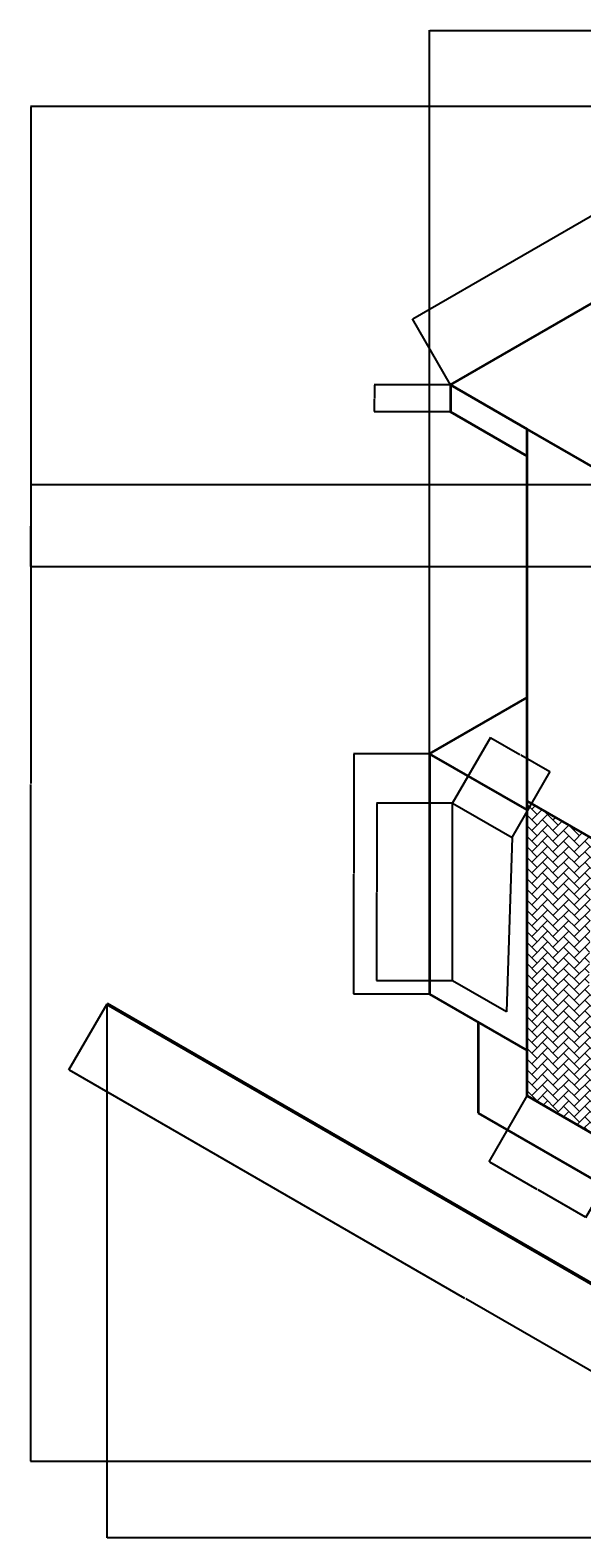
# Model space of a CAD drawing. Units: inches. Extents: x 61 to 939, y -128 to 676.
# Tile 1 of 3: x 61 to 355, y -128 to 676. Entities that reach past the tile are written whole.
import ezdxf

# ---------------------------------------------------------------- set-up
doc = ezdxf.new("R2010")
doc.units = ezdxf.units.IN
doc.header["$MEASUREMENT"] = 0
for name, color, linetype, lineweight in [('A-ANNO-DIMS', 2, 'Continuous', 18), ('A-ELEV', 7, 'Continuous', 35), ('A-GLAZ', 4, 'Continuous', 25), ('A-WALL-PATT', 8, 'Continuous', 18), ('C-TOPO', 7, 'Continuous', 50)]:
    doc.layers.add(name, color=color, linetype=linetype, lineweight=lineweight)
doc.styles.get("Standard").update_dxf_attribs({"font": 'arial.ttf'})
doc.dimstyles.get("Standard").update_dxf_attribs({"dimtxt": 0.18, "dimasz": 0.18, "dimexe": 0.18, "dimexo": 0.0625, "dimgap": 0.09, "dimtad": 0, "dimtih": 1, "dimtoh": 1, "dimdec": 4, "dimzin": 0, "dimdsep": 46, "dimtxsty": 'Standard', "dimcen": 0.09, "dimadec": 0, "dimazin": 0, "dimtfac": 1, "dimtdec": 4, "dimtofl": 0, "dimtmove": 0, "dimatfit": 3, "dimfxl": 1, "dimtolj": 1, "dimtzin": 0, "dimarcsym": 0})

# ---------------------------------------------------------------- blocks, each defined once
blk = doc.blocks.new('*D1')
at = {"layer": 'A-ANNO-DIMS', "color": 0, "lineweight": -2, "transparency": 16777216}
for p, q in [((273.62, 289.95), (273.62, 675.84)), ((273.8, 675.66), (542.03, 675.66)), ((811.05, 675.66), (542.82, 675.66)), ((811.23, 479.78), (811.23, 675.84))]:
    blk.add_line(p, q, dxfattribs=at)
at = {"layer": 'A-ANNO-DIMS', "color": 0, "transparency": 16777216}
for points in [[(273.8, 675.69), (273.8, 675.63), (273.62, 675.66)], [(811.05, 675.69), (811.05, 675.63), (811.23, 675.66)]]:
    blk.add_solid(points, dxfattribs=at)
at = {"layer": 'Defpoints', "color": 0, "transparency": 16777216}
for p in [(811.23, 675.66), (811.23, 479.72), (273.62, 289.89)]:
    blk.add_point(p, dxfattribs=at)
at = {"layer": 'A-ANNO-DIMS', "color": 0, "transparency": 16777216, "insert": (542.42, 675.66), "char_height": 0.18, "attachment_point": 5}
blk.add_mtext('\\A1;537.6', dxfattribs=at)
blk = doc.blocks.new('*D2')
at = {"layer": 'A-ANNO-DIMS', "color": 0, "lineweight": -2, "transparency": 16777216}
for p, q in [((541.93, 635.16), (60.74, 635.16)), ((60.92, 634.98), (60.92, 273.9)), ((60.92, -87.54), (60.92, 273.54)), ((524.15, -87.72), (60.74, -87.72))]:
    blk.add_line(p, q, dxfattribs=at)
at = {"layer": 'A-ANNO-DIMS', "color": 0, "transparency": 16777216}
for points in [[(60.89, 634.98), (60.95, 634.98), (60.92, 635.16)], [(60.89, -87.54), (60.95, -87.54), (60.92, -87.72)]]:
    blk.add_solid(points, dxfattribs=at)
at = {"layer": 'Defpoints', "color": 0, "transparency": 16777216}
for p in [(60.92, 635.16), (542, 635.16), (524.21, -87.72)]:
    blk.add_point(p, dxfattribs=at)
at = {"layer": 'A-ANNO-DIMS', "color": 0, "transparency": 16777216, "insert": (60.92, 273.72), "char_height": 0.18, "attachment_point": 5}
blk.add_mtext('\\A1;722.9', dxfattribs=at)
blk = doc.blocks.new('*D3')
at = {"layer": 'A-ANNO-DIMS', "color": 0, "lineweight": -2, "transparency": 16777216}
for p, q in [((101.42, 156.32), (101.42, -128.4)), ((897.89, 127.95), (897.89, -128.4)), ((101.6, -128.22), (499.26, -128.22)), ((897.71, -128.22), (500.04, -128.22))]:
    blk.add_line(p, q, dxfattribs=at)
at = {"layer": 'A-ANNO-DIMS', "color": 0, "transparency": 16777216}
for points in [[(101.6, -128.19), (101.6, -128.25), (101.42, -128.22)], [(897.71, -128.19), (897.71, -128.25), (897.89, -128.22)]]:
    blk.add_solid(points, dxfattribs=at)
at = {"layer": 'Defpoints', "color": 0, "transparency": 16777216}
for p in [(101.42, 156.38), (897.89, 128.02), (897.89, -128.22)]:
    blk.add_point(p, dxfattribs=at)
at = {"layer": 'A-ANNO-DIMS', "color": 0, "transparency": 16777216, "insert": (499.65, -128.22), "char_height": 0.18, "attachment_point": 5}
blk.add_mtext('\\A1;796.5', dxfattribs=at)
blk = doc.blocks.new('*D9')
at = {"layer": 'A-ANNO-DIMS', "color": 0, "lineweight": -2, "transparency": 16777216}
for p, q in [((273.55, 289.89), (232.94, 289.89)), ((233.12, 289.71), (233.12, 225.93)), ((233.12, 161.78), (233.12, 225.56)), ((273.55, 161.6), (232.94, 161.6))]:
    blk.add_line(p, q, dxfattribs=at)
at = {"layer": 'A-ANNO-DIMS', "color": 0, "transparency": 16777216}
for points in [[(233.09, 289.71), (233.15, 289.71), (233.12, 289.89)], [(233.09, 161.78), (233.15, 161.78), (233.12, 161.6)]]:
    blk.add_solid(points, dxfattribs=at)
at = {"layer": 'Defpoints', "color": 0, "transparency": 16777216}
for p in [(233.12, 289.89), (273.62, 289.89), (273.62, 161.6)]:
    blk.add_point(p, dxfattribs=at)
at = {"layer": 'A-ANNO-DIMS', "color": 0, "transparency": 16777216, "insert": (233.12, 225.74), "char_height": 0.18, "attachment_point": 5}
blk.add_mtext('\\A1;128.28', dxfattribs=at)
blk = doc.blocks.new('*D10')
at = {"layer": 'A-ANNO-DIMS', "color": 0, "lineweight": -2, "transparency": 16777216}
for p, q in [((284.69, 486.64), (244.07, 486.64)), ((244.25, 486.46), (244.25, 479.61)), ((244.25, 472.4), (244.25, 479.25)), ((284.69, 472.22), (244.07, 472.22))]:
    blk.add_line(p, q, dxfattribs=at)
at = {"layer": 'A-ANNO-DIMS', "color": 0, "transparency": 16777216}
for points in [[(244.22, 486.46), (244.28, 486.46), (244.25, 486.64)], [(244.22, 472.4), (244.28, 472.4), (244.25, 472.22)]]:
    blk.add_solid(points, dxfattribs=at)
at = {"layer": 'Defpoints', "color": 0, "transparency": 16777216}
for p in [(244.25, 486.64), (284.75, 486.64), (284.75, 472.22)]:
    blk.add_point(p, dxfattribs=at)
at = {"layer": 'A-ANNO-DIMS', "color": 0, "transparency": 16777216, "insert": (244.25, 479.43), "char_height": 0.18, "attachment_point": 5}
blk.add_mtext('\\A1;14.418', dxfattribs=at)
blk = doc.blocks.new('*D18')
at = {"layer": 'A-ANNO-DIMS', "color": 0, "lineweight": -2, "transparency": 16777216}
for p, q in [((285.81, 263.41), (245.2, 263.41)), ((245.38, 263.23), (245.38, 216.27)), ((245.38, 168.94), (245.38, 215.9)), ((285.81, 168.76), (245.2, 168.76))]:
    blk.add_line(p, q, dxfattribs=at)
at = {"layer": 'A-ANNO-DIMS', "color": 0, "transparency": 16777216}
for points in [[(245.35, 263.23), (245.41, 263.23), (245.38, 263.41)], [(245.35, 168.94), (245.41, 168.94), (245.38, 168.76)]]:
    blk.add_solid(points, dxfattribs=at)
at = {"layer": 'Defpoints', "color": 0, "transparency": 16777216}
for p in [(245.38, 263.41), (285.88, 263.41), (285.88, 168.76)]:
    blk.add_point(p, dxfattribs=at)
at = {"layer": 'A-ANNO-DIMS', "color": 0, "transparency": 16777216, "insert": (245.38, 216.09), "char_height": 0.18, "attachment_point": 5}
blk.add_mtext('\\A1;94.65', dxfattribs=at)
blk = doc.blocks.new('*D19')
at = {"layer": 'A-ANNO-DIMS', "color": 0, "lineweight": -2, "transparency": 16777216}
for p, q in [((285.91, 263.47), (306.22, 298.64)), ((306.28, 298.4), (321.66, 289.52)), ((337.66, 280.28), (322.29, 289.16)), ((317.6, 245.17), (337.91, 280.35))]:
    blk.add_line(p, q, dxfattribs=at)
at = {"layer": 'A-ANNO-DIMS', "color": 0, "transparency": 16777216}
for points in [[(306.3, 298.42), (306.27, 298.37), (306.13, 298.49)], [(337.68, 280.31), (337.65, 280.25), (337.82, 280.19)]]:
    blk.add_solid(points, dxfattribs=at)
at = {"layer": 'Defpoints', "color": 0, "transparency": 16777216}
for p in [(337.82, 280.19), (285.88, 263.41), (317.57, 245.12)]:
    blk.add_point(p, dxfattribs=at)
at = {"layer": 'A-ANNO-DIMS', "color": 0, "transparency": 16777216, "insert": (321.97, 289.34), "char_height": 0.18, "attachment_point": 5}
blk.add_mtext('\\A1;36.59', dxfattribs=at)
blk = doc.blocks.new('*D26')
at = {"layer": 'A-ANNO-DIMS', "color": 0, "lineweight": -2, "transparency": 16777216}
for p, q in [((101.38, 156.32), (81.08, 121.15)), ((81.32, 121.21), (292.25, -0.57)), ((503.81, -122.71), (292.88, -0.93)), ((524.18, -87.78), (503.87, -122.95))]:
    blk.add_line(p, q, dxfattribs=at)
at = {"layer": 'A-ANNO-DIMS', "color": 0, "transparency": 16777216}
for points in [[(81.34, 121.24), (81.31, 121.19), (81.17, 121.3)], [(503.82, -122.68), (503.79, -122.73), (503.96, -122.8)]]:
    blk.add_solid(points, dxfattribs=at)
at = {"layer": 'Defpoints', "color": 0, "transparency": 16777216}
for p in [(101.42, 156.38), (81.17, 121.3), (524.21, -87.72)]:
    blk.add_point(p, dxfattribs=at)
at = {"layer": 'A-ANNO-DIMS', "color": 0, "transparency": 16777216, "insert": (292.56, -0.75), "char_height": 0.18, "attachment_point": 5}
blk.add_mtext('\\A1;488.20', dxfattribs=at)
blk = doc.blocks.new('*D28')
at = {"layer": 'A-ANNO-DIMS', "color": 0, "lineweight": -2, "transparency": 16777216}
for p, q in [((521.59, 670.14), (393.44, 596.16)), ((541.96, 635.21), (521.66, 670.39)), ((264.66, 521.8), (392.81, 595.79)), ((284.72, 486.69), (264.41, 521.87))]:
    blk.add_line(p, q, dxfattribs=at)
at = {"layer": 'A-ANNO-DIMS', "color": 0, "transparency": 16777216}
for points in [[(521.57, 670.17), (521.6, 670.12), (521.75, 670.23)], [(264.64, 521.83), (264.67, 521.78), (264.5, 521.71)]]:
    blk.add_solid(points, dxfattribs=at)
at = {"layer": 'Defpoints', "color": 0, "transparency": 16777216}
for p in [(521.75, 670.23), (542, 635.16), (284.75, 486.64)]:
    blk.add_point(p, dxfattribs=at)
at = {"layer": 'A-ANNO-DIMS', "color": 0, "transparency": 16777216, "insert": (393.12, 595.97), "char_height": 0.18, "attachment_point": 5}
blk.add_mtext('\\A1;297.04', dxfattribs=at)
blk = doc.blocks.new('*D32')
at = {"layer": 'A-ANNO-DIMS', "color": 0, "lineweight": -2, "transparency": 16777216}
for p, q in [((623.49, 433.3), (60.74, 433.3)), ((60.92, 433.12), (60.92, 411.64)), ((60.92, 389.79), (60.92, 411.27)), ((623.49, 389.61), (60.74, 389.61))]:
    blk.add_line(p, q, dxfattribs=at)
at = {"layer": 'A-ANNO-DIMS', "color": 0, "transparency": 16777216}
for points in [[(60.89, 433.12), (60.95, 433.12), (60.92, 433.3)], [(60.89, 389.79), (60.95, 389.79), (60.92, 389.61)]]:
    blk.add_solid(points, dxfattribs=at)
at = {"layer": 'Defpoints', "color": 0, "transparency": 16777216}
for p in [(623.55, 433.3), (60.92, 389.61), (623.55, 389.61)]:
    blk.add_point(p, dxfattribs=at)
at = {"layer": 'A-ANNO-DIMS', "color": 0, "transparency": 16777216, "insert": (60.92, 411.46), "char_height": 0.18, "attachment_point": 5}
blk.add_mtext('\\A1;43.695', dxfattribs=at)
blk = doc.blocks.new('*D37')
at = {"layer": 'A-ANNO-DIMS', "color": 0, "lineweight": -2, "transparency": 16777216}
for p, q in [((325.55, 107.3), (305.24, 72.12)), ((377.15, 77.51), (356.84, 42.33)), ((305.48, 72.19), (330.81, 57.56)), ((356.77, 42.58), (331.44, 57.2))]:
    blk.add_line(p, q, dxfattribs=at)
at = {"layer": 'A-ANNO-DIMS', "color": 0, "transparency": 16777216}
for points in [[(305.5, 72.21), (305.47, 72.16), (305.33, 72.28)], [(356.79, 42.6), (356.76, 42.55), (356.93, 42.49)]]:
    blk.add_solid(points, dxfattribs=at)
at = {"layer": 'Defpoints', "color": 0, "transparency": 16777216}
for p in [(325.58, 107.35), (377.18, 77.56), (305.33, 72.28)]:
    blk.add_point(p, dxfattribs=at)
at = {"layer": 'A-ANNO-DIMS', "color": 0, "transparency": 16777216, "insert": (331.13, 57.38), "char_height": 0.18, "attachment_point": 5}
blk.add_mtext('\\A1;59.58', dxfattribs=at)

msp = doc.modelspace()

# ---------------------------------------------------------------- hatches: boundary and pattern name
at = {"layer": 'A-WALL-PATT'}
h = msp.add_hatch(dxfattribs=at)
h.set_pattern_fill('AR-HBONE', color=256)
h.paths.add_polyline_path([(764.8272, 163.8587), (764.8272, 294.6874), (562.2436, 177.7257), (562.2436, 46.897)])
h.paths.add_polyline_path([(595.2101, 166.7105), (749.5189, 260.1923), (749.5189, 172.9507), (595.1042, 87.0956)], flags=16)
h.paths.add_polyline_path([(377.1796, 153.7437), (358.6559, 164.4384), (359.9295, 244.7895), (325.5788, 264.6219), (325.5788, 215.6029), (325.5788, 131.6029), (325.5788, 107.3524), (377.1796, 77.5607)])

# ---------------------------------------------------------------- linework, layer by layer
at = {"layer": 'A-ELEV'}
for p, q in [((284.7507, 486.6398), (541.9952, 635.1599)), ((325.5788, 463.0676), (284.7507, 486.6398)), ((284.7507, 486.6398), (284.7507, 472.2218)), ((284.7507, 472.2218), (325.5788, 448.6497)), ((325.5788, 215.6029), (325.5788, 463.0676)), ((504.1826, 359.9507), (325.5788, 463.0676)), ((273.6173, 289.886), (325.5788, 319.886)), ((325.5788, 259.886), (273.6173, 289.886)), ((273.6173, 289.886), (273.6173, 161.6029)), ((325.5788, 264.6219), (383.2216, 231.3418)), ((325.5788, 131.6029), (325.5788, 215.6029)), ((273.6173, 161.6029), (325.5788, 131.6029)), ((299.5981, 146.6029), (299.5981, 98.102)), ((325.5788, 107.3524), (325.5788, 131.6029)), ((377.1796, 77.5607), (325.5788, 107.3524)), ((299.5981, 98.102), (403.5211, 38.102))]:
    msp.add_line(p, q, dxfattribs=at)
at = {"layer": 'A-GLAZ'}
for p, q in [((285.8771, 168.7602), (285.8771, 263.4127)), ((285.8771, 263.4127), (317.568, 245.116)), ((317.568, 245.116), (314.5549, 152.2031)), ((314.5549, 152.2031), (285.8771, 168.7602))]:
    msp.add_line(p, q, dxfattribs=at)
at = {"layer": 'C-TOPO'}
msp.add_line((524.212, -87.7241), (101.4156, 156.3775), dxfattribs=at)

# ---------------------------------------------------------------- dimensions: what is measured, and where the dimension line sits
at = {"layer": 'A-ANNO-DIMS'}
for base, p1, p2, picture, middle in [((811.2295, 675.6599), (273.6173, 289.886), (811.2295, 479.7174), '*D1', (542.4234, 675.6599)), ((897.8863, -128.2241), (101.4156, 156.3775), (897.8863, 128.0168), '*D3', (499.6509, -128.2241))]:
    dim = msp.add_linear_dim(base=base, p1=p1, p2=p2, dimstyle='Standard', override={"dimdec": 1, "dimlfac": 1, "dimrnd": 0, "dimzin": 0, "dimdsep": 46, "dimlunit": 2}, dxfattribs=at)
    dim.commit()
    dim.dimension.update_dxf_attribs({"geometry": picture, "text_midpoint": middle})
for base, p1, p2, angle, override, picture, middle in [((521.7452, 670.2339), (284.7507, 486.6398), (541.9952, 635.1599), 30, {"dimdec": 2, "dimlfac": 1, "dimrnd": 0, "dimzin": 0, "dimdsep": 46, "dimlunit": 2}, '*D28', (393.1229, 595.9738)), ((60.9156, 635.1599), (524.212, -87.7241), (541.9952, 635.1599), 90, {"dimdec": 1, "dimlfac": 1, "dimrnd": 0, "dimzin": 0, "dimdsep": 46, "dimlunit": 2}, '*D2', (60.9156, 273.7179)), ((244.2507, 486.6398), (284.7507, 472.2218), (284.7507, 486.6398), 90, {"dimdec": 3, "dimlfac": 1, "dimrnd": 0, "dimzin": 0, "dimdsep": 46, "dimlunit": 2}, '*D10', (244.2507, 479.4308)), ((60.9156, 389.6079), (623.5481, 433.303), (623.5481, 389.6079), 90, {"dimdec": 3, "dimlfac": 1, "dimrnd": 0, "dimzin": 0, "dimdsep": 46, "dimlunit": 2}, '*D32', (60.9156, 411.4554)), ((337.818, 280.1901), (285.8771, 263.4127), (317.568, 245.116), 330, {"dimdec": 2, "dimlfac": 1, "dimrnd": 0, "dimzin": 0, "dimdsep": 46, "dimlunit": 2}, '*D19', (321.9726, 289.3384)), ((233.1173, 289.886), (273.6173, 161.6029), (273.6173, 289.886), 90, {"dimdec": 2, "dimlfac": 1, "dimrnd": 0, "dimzin": 0, "dimdsep": 46, "dimlunit": 2}, '*D9', (233.1173, 225.7444)), ((245.3771, 263.4127), (285.8771, 168.7602), (285.8771, 263.4127), 90, {"dimdec": 2, "dimlfac": 1, "dimrnd": 0, "dimzin": 0, "dimdsep": 46, "dimlunit": 2}, '*D18', (245.3771, 216.0865)), ((81.1656, 121.3035), (524.212, -87.7241), (101.4156, 156.3775), 150, {"dimdec": 2, "dimlfac": 1, "dimrnd": 0, "dimzin": 0, "dimdsep": 46, "dimlunit": 2}, '*D26', (292.5638, -0.7473)), ((305.3288, 72.2784), (377.1796, 77.5607), (325.5788, 107.3524), 150, {"dimdec": 2, "dimlfac": 1, "dimrnd": 0, "dimzin": 0, "dimdsep": 46, "dimlunit": 2}, '*D37', (331.1292, 57.3825))]:
    dim = msp.add_linear_dim(base=base, p1=p1, p2=p2, angle=angle, dimstyle='Standard', override=override, dxfattribs=at)
    dim.commit()
    dim.dimension.update_dxf_attribs({"geometry": picture, "text_midpoint": middle})

doc.saveas('drawing.dxf')
